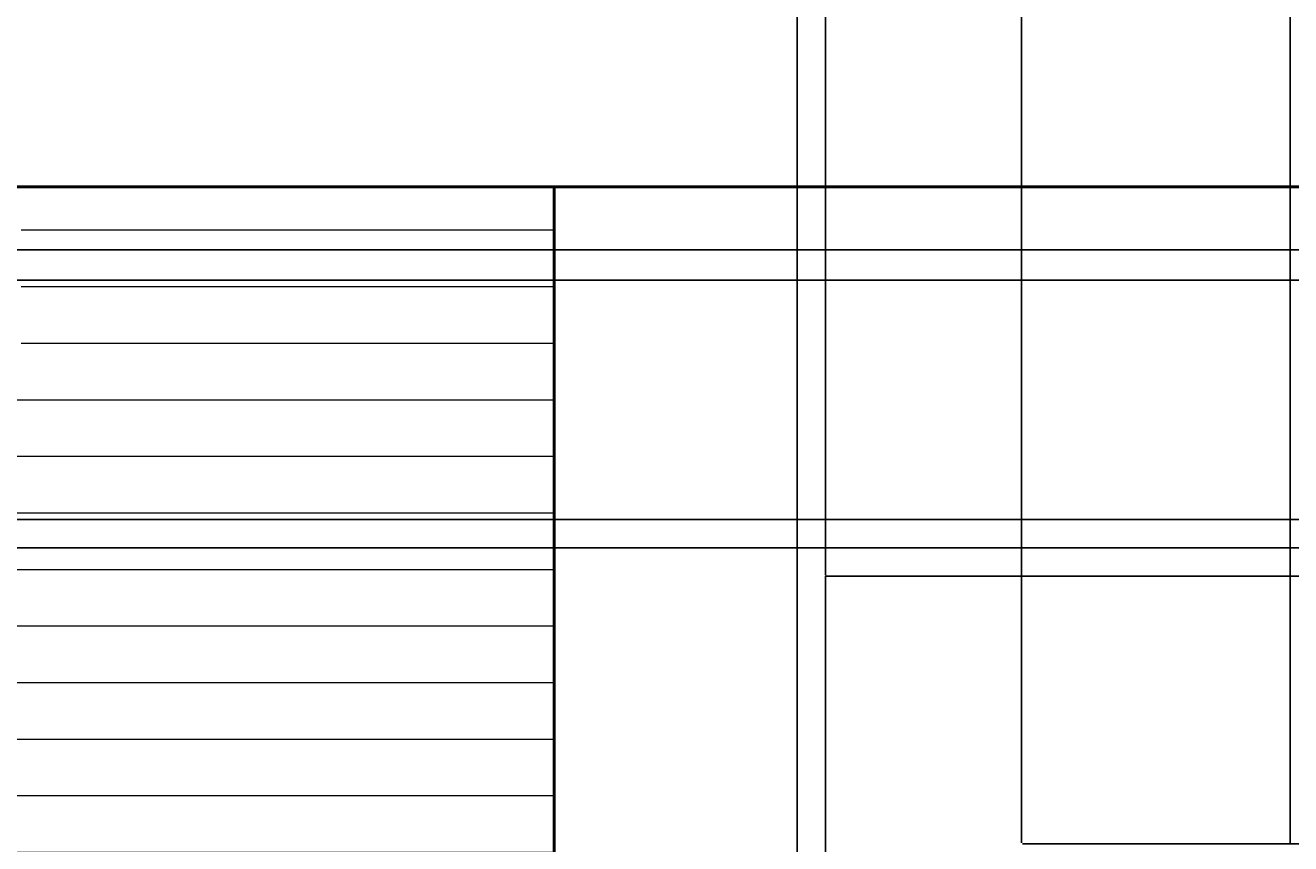
# Model space of a CAD drawing. Units: inches. Extents: x -139 to 346, y 72 to 413.
# Tile 12 of 18: x 175 to 265, y 185 to 242. Entities that reach past the tile are written whole.
import ezdxf

# ---------------------------------------------------------------- set-up
doc = ezdxf.new("R2010")
doc.units = ezdxf.units.IN
doc.header["$MEASUREMENT"] = 0
for name, color, linetype, lineweight in [('A-ANNO-DIMS', 2, 'Continuous', 18), ('A-DOOR', 3, 'Continuous', 25), ('A-WALL', 7, 'Continuous', 50), ('A-WALL-PATT', 8, 'Continuous', 13)]:
    doc.layers.add(name, color=color, linetype=linetype, lineweight=lineweight)
doc.styles.get("Standard").update_dxf_attribs({"font": 'arial.ttf'})
doc.dimstyles.get("Standard").update_dxf_attribs({"dimtxt": 0.6875, "dimasz": 0.18, "dimexe": 0.18, "dimexo": 0.0625, "dimgap": 0.09, "dimtad": 0, "dimtih": 1, "dimtoh": 1, "dimdec": 4, "dimzin": 0, "dimdsep": 46, "dimlunit": 4, "dimtxsty": 'Standard', "dimcen": 0.09, "dimadec": 0, "dimazin": 0, "dimtfac": 1, "dimtdec": 4, "dimtofl": 0, "dimtmove": 0, "dimatfit": 3, "dimfxl": 1, "dimtolj": 1, "dimtzin": 0, "dimarcsym": 0})

# ---------------------------------------------------------------- blocks, each defined once
blk = doc.blocks.new('*D54')
at = {"layer": 'A-ANNO-DIMS', "color": 0, "lineweight": -2, "transparency": 16777216}
for p, q in [((-47.211, 224.459), (344.386, 224.459)), ((344.206, 224.279), (344.206, 216.433)), ((344.206, 207.704), (344.206, 215.55)), ((-47.211, 207.524), (344.386, 207.524))]:
    blk.add_line(p, q, dxfattribs=at)
at = {"layer": 'A-ANNO-DIMS', "color": 0, "transparency": 16777216}
for points in [[(344.176, 224.279), (344.236, 224.279), (344.206, 224.459)], [(344.176, 207.704), (344.236, 207.704), (344.206, 207.524)]]:
    blk.add_solid(points, dxfattribs=at)
at = {"layer": 'Defpoints', "color": 0, "transparency": 16777216}
for p in [(-47.273, 224.459), (344.206, 224.459), (-47.273, 207.524)]:
    blk.add_point(p, dxfattribs=at)
at = {"layer": 'A-ANNO-DIMS', "color": 0, "transparency": 16777216, "insert": (344.206, 215.992), "char_height": 0.6875, "attachment_point": 5}
blk.add_mtext('\\A1;16.935', dxfattribs=at)
blk = doc.blocks.new('*D55')
at = {"layer": 'A-ANNO-DIMS', "color": 0, "lineweight": -2, "transparency": 16777216}
for p, q in [((-47.211, 226.606), (344.386, 226.606)), ((344.206, 226.426), (344.206, 225.968)), ((344.206, 224.639), (344.206, 225.097)), ((-47.211, 224.459), (344.386, 224.459))]:
    blk.add_line(p, q, dxfattribs=at)
at = {"layer": 'A-ANNO-DIMS', "color": 0, "transparency": 16777216}
for points in [[(344.176, 226.426), (344.236, 226.426), (344.206, 226.606)], [(344.176, 224.639), (344.236, 224.639), (344.206, 224.459)]]:
    blk.add_solid(points, dxfattribs=at)
at = {"layer": 'Defpoints', "color": 0, "transparency": 16777216}
for p in [(-47.273, 226.606), (344.206, 226.606), (-47.273, 224.459)]:
    blk.add_point(p, dxfattribs=at)
at = {"layer": 'A-ANNO-DIMS', "color": 0, "transparency": 16777216, "insert": (344.206, 225.533), "char_height": 0.6875, "attachment_point": 5}
blk.add_mtext('\\A1;2.147', dxfattribs=at)
blk = doc.blocks.new('*D65')
at = {"layer": 'A-ANNO-DIMS', "color": 0, "lineweight": -2, "transparency": 16777216}
for p, q in [((55.328, 205.524), (344.386, 205.524)), ((344.206, 205.344), (344.206, 178.581)), ((344.206, 150.938), (344.206, 177.701)), ((55.328, 150.758), (344.386, 150.758))]:
    blk.add_line(p, q, dxfattribs=at)
at = {"layer": 'A-ANNO-DIMS', "color": 0, "transparency": 16777216}
for points in [[(344.176, 205.344), (344.236, 205.344), (344.206, 205.524)], [(344.176, 150.938), (344.236, 150.938), (344.206, 150.758)]]:
    blk.add_solid(points, dxfattribs=at)
at = {"layer": 'Defpoints', "color": 0, "transparency": 16777216}
for p in [(55.265, 205.524), (344.206, 205.524), (55.265, 150.758)]:
    blk.add_point(p, dxfattribs=at)
at = {"layer": 'A-ANNO-DIMS', "color": 0, "transparency": 16777216, "insert": (344.206, 178.141), "char_height": 0.6875, "attachment_point": 5}
blk.add_mtext('\\A1;54.77', dxfattribs=at)
blk = doc.blocks.new('*D66')
at = {"layer": 'A-ANNO-DIMS', "color": 0, "lineweight": -2, "transparency": 16777216}
for p, q in [((57.328, 207.524), (344.386, 207.524)), ((344.206, 207.344), (344.206, 206.96)), ((344.206, 205.704), (344.206, 206.089)), ((55.328, 205.524), (344.386, 205.524))]:
    blk.add_line(p, q, dxfattribs=at)
at = {"layer": 'A-ANNO-DIMS', "color": 0, "transparency": 16777216}
for points in [[(344.176, 207.344), (344.236, 207.344), (344.206, 207.524)], [(344.176, 205.704), (344.236, 205.704), (344.206, 205.524)]]:
    blk.add_solid(points, dxfattribs=at)
at = {"layer": 'Defpoints', "color": 0, "transparency": 16777216}
for p in [(57.265, 207.524), (344.206, 207.524), (55.265, 205.524)]:
    blk.add_point(p, dxfattribs=at)
at = {"layer": 'A-ANNO-DIMS', "color": 0, "transparency": 16777216, "insert": (344.206, 206.524), "char_height": 0.6875, "attachment_point": 5}
blk.add_mtext('\\A1;2', dxfattribs=at)
blk = doc.blocks.new('*D67')
at = {"layer": 'A-ANNO-DIMS', "color": 0, "lineweight": -2, "transparency": 16777216}
for p, q in [((57.328, 207.524), (344.386, 207.524)), ((344.206, 207.344), (344.206, 165.091)), ((344.206, 121.955), (344.206, 164.209)), ((57.328, 121.775), (344.386, 121.775))]:
    blk.add_line(p, q, dxfattribs=at)
at = {"layer": 'A-ANNO-DIMS', "color": 0, "transparency": 16777216}
for points in [[(344.176, 207.344), (344.236, 207.344), (344.206, 207.524)], [(344.176, 121.955), (344.236, 121.955), (344.206, 121.775)]]:
    blk.add_solid(points, dxfattribs=at)
at = {"layer": 'Defpoints', "color": 0, "transparency": 16777216}
for p in [(57.265, 207.524), (344.206, 207.524), (57.265, 121.775)]:
    blk.add_point(p, dxfattribs=at)
at = {"layer": 'A-ANNO-DIMS', "color": 0, "transparency": 16777216, "insert": (344.206, 164.65), "char_height": 0.6875, "attachment_point": 5}
blk.add_mtext('\\A1;85.75', dxfattribs=at)
blk = doc.blocks.new('*D80')
at = {"layer": 'A-ANNO-DIMS', "color": 0, "lineweight": -2, "transparency": 16777216}
for p, q in [((229.972, 205.587), (229.972, 412.455)), ((230.152, 412.275), (230.654, 412.275)), ((231.792, 412.275), (231.29, 412.275)), ((231.972, 203.587), (231.972, 412.455))]:
    blk.add_line(p, q, dxfattribs=at)
at = {"layer": 'A-ANNO-DIMS', "color": 0, "transparency": 16777216}
for points in [[(230.152, 412.305), (230.152, 412.245), (229.972, 412.275)], [(231.792, 412.305), (231.792, 412.245), (231.972, 412.275)]]:
    blk.add_solid(points, dxfattribs=at)
at = {"layer": 'Defpoints', "color": 0, "transparency": 16777216}
for p in [(231.972, 412.275), (229.972, 205.524), (231.972, 203.524)]:
    blk.add_point(p, dxfattribs=at)
at = {"layer": 'A-ANNO-DIMS', "color": 0, "transparency": 16777216, "insert": (230.972, 412.275), "char_height": 0.6875, "attachment_point": 5}
blk.add_mtext('\\A1;2', dxfattribs=at)
blk = doc.blocks.new('*D81')
at = {"layer": 'A-ANNO-DIMS', "color": 0, "lineweight": -2, "transparency": 16777216}
for p, q in [((231.972, 203.587), (231.972, 412.455)), ((232.152, 412.275), (237.421, 412.275)), ((245.66, 412.275), (240.391, 412.275)), ((245.84, 184.668), (245.84, 412.455))]:
    blk.add_line(p, q, dxfattribs=at)
at = {"layer": 'A-ANNO-DIMS', "color": 0, "transparency": 16777216}
for points in [[(232.152, 412.305), (232.152, 412.245), (231.972, 412.275)], [(245.66, 412.305), (245.66, 412.245), (245.84, 412.275)]]:
    blk.add_solid(points, dxfattribs=at)
at = {"layer": 'Defpoints', "color": 0, "transparency": 16777216}
for p in [(245.84, 412.275), (231.972, 203.524), (245.84, 184.606)]:
    blk.add_point(p, dxfattribs=at)
at = {"layer": 'A-ANNO-DIMS', "color": 0, "transparency": 16777216, "insert": (238.906, 412.275), "char_height": 0.6875, "attachment_point": 5}
blk.add_mtext('\\A1;13.868', dxfattribs=at)
blk = doc.blocks.new('*D82')
at = {"layer": 'A-ANNO-DIMS', "color": 0, "lineweight": -2, "transparency": 16777216}
for p, q in [((245.84, 184.668), (245.84, 412.455)), ((246.02, 412.275), (253.85, 412.275)), ((264.642, 412.275), (256.812, 412.275)), ((264.822, 184.668), (264.822, 412.455))]:
    blk.add_line(p, q, dxfattribs=at)
at = {"layer": 'A-ANNO-DIMS', "color": 0, "transparency": 16777216}
for points in [[(246.02, 412.305), (246.02, 412.245), (245.84, 412.275)], [(264.642, 412.305), (264.642, 412.245), (264.822, 412.275)]]:
    blk.add_solid(points, dxfattribs=at)
at = {"layer": 'Defpoints', "color": 0, "transparency": 16777216}
for p in [(264.822, 412.275), (245.84, 184.606), (264.822, 184.606)]:
    blk.add_point(p, dxfattribs=at)
at = {"layer": 'A-ANNO-DIMS', "color": 0, "transparency": 16777216, "insert": (255.331, 412.275), "char_height": 0.6875, "attachment_point": 5}
blk.add_mtext('\\A1;18.982', dxfattribs=at)
blk = doc.blocks.new('*D84')
at = {"layer": 'A-ANNO-DIMS', "color": 0, "lineweight": -2, "transparency": 16777216}
for p, q in [((245.902, 184.606), (344.386, 184.606)), ((344.206, 184.426), (344.206, 153.665)), ((344.206, 122.023), (344.206, 152.783)), ((245.902, 121.843), (344.386, 121.843))]:
    blk.add_line(p, q, dxfattribs=at)
at = {"layer": 'A-ANNO-DIMS', "color": 0, "transparency": 16777216}
for points in [[(344.176, 184.426), (344.236, 184.426), (344.206, 184.606)], [(344.176, 122.023), (344.236, 122.023), (344.206, 121.843)]]:
    blk.add_solid(points, dxfattribs=at)
at = {"layer": 'Defpoints', "color": 0, "transparency": 16777216}
for p in [(245.84, 184.606), (344.206, 184.606), (245.84, 121.843)]:
    blk.add_point(p, dxfattribs=at)
at = {"layer": 'A-ANNO-DIMS', "color": 0, "transparency": 16777216, "insert": (344.206, 153.224), "char_height": 0.6875, "attachment_point": 5}
blk.add_mtext('\\A1;62.76', dxfattribs=at)

msp = doc.modelspace()

# ---------------------------------------------------------------- hatches: boundary and pattern name
at = {"layer": 'A-WALL-PATT'}
h = msp.add_hatch(dxfattribs=at)
h.set_pattern_fill('ANSI31', color=256, scale=32, angle=135)
h.paths.add_polyline_path([(98.6724, 360.5443), (-34.7346, 360.5443), (-34.7346, 353.0644), (-34.7346, 305.9205), (5.6729, 305.9205), (5.6729, 338.3217), (62.4258, 338.3217), (62.4258, 305.9205), (98.6724, 305.9205)])
h.paths.add_polyline_path([(212.769, 231.0607), (175.072, 231.0607), (175.072, 218.0635), (171.0337, 218.0635), (171.0337, 115.6761), (125.2464, 115.6761), (125.2464, 218.0635), (123.4318, 218.0635), (120.5054, 218.0635), (120.5054, 231.0607), (112.6506, 231.0607), (112.6506, 112.6042), (212.769, 112.6042)])

# ---------------------------------------------------------------- linework, layer by layer
at = {"layer": 'A-DOOR'}
for points in [[(229.972, 205.5243), (283.8497, 205.5243), (283.8497, 104.5429), (229.972, 104.5429)], [(231.972, 203.5243), (281.8497, 203.5243), (281.8497, 106.5429), (231.972, 106.5429)]]:
    msp.add_lwpolyline(points, close=True, dxfattribs=at)
at = {"layer": 'A-WALL'}
for p, q in [((297.5013, 231.0607), (112.6506, 231.0607)), ((212.769, 231.0607), (212.769, 94.9748))]:
    msp.add_line(p, q, dxfattribs=at)

# ---------------------------------------------------------------- dimensions: what is measured, and where the dimension line sits
at = {"layer": 'A-ANNO-DIMS'}
for base, p1, p2, override, picture, middle in [((231.972, 412.2748), (229.972, 205.5243), (231.972, 203.5243), {"dimdec": 0, "dimlfac": 1, "dimrnd": 0, "dimzin": 0, "dimdsep": 46, "dimlunit": 2}, '*D80', (230.972, 412.2748)), ((245.8399, 412.2748), (231.972, 203.5243), (245.8399, 184.6055), {"dimdec": 3, "dimlfac": 1, "dimrnd": 0, "dimzin": 0, "dimdsep": 46, "dimlunit": 2}, '*D81', (238.906, 412.2748)), ((264.8219, 412.2748), (245.8399, 184.6055), (264.8219, 184.6055), {"dimdec": 3, "dimlfac": 1, "dimrnd": 0, "dimzin": 0, "dimdsep": 46, "dimlunit": 2}, '*D82', (255.3309, 412.2748))]:
    dim = msp.add_linear_dim(base=base, p1=p1, p2=p2, dimstyle='Standard', override=override, dxfattribs=at)
    dim.commit()
    dim.dimension.update_dxf_attribs({"geometry": picture, "text_midpoint": middle})
for base, p1, p2, override, picture, middle in [((344.2055, 226.6062), (-47.2734, 224.4591), (-47.2734, 226.6062), {"dimdec": 3, "dimlfac": 1, "dimrnd": 0, "dimzin": 0, "dimdsep": 46, "dimlunit": 2}, '*D55', (344.2055, 225.5327)), ((344.2055, 224.4591), (-47.2734, 207.5243), (-47.2734, 224.4591), {"dimdec": 3, "dimlfac": 1, "dimrnd": 0, "dimzin": 0, "dimdsep": 46, "dimlunit": 2}, '*D54', (344.2055, 215.9917)), ((344.2055, 207.5243), (55.2654, 205.5243), (57.2654, 207.5243), {"dimdec": 0, "dimlfac": 1, "dimrnd": 0, "dimzin": 0, "dimdsep": 46, "dimlunit": 2}, '*D66', (344.2055, 206.5243)), ((344.2055, 207.5243), (57.2654, 121.7753), (57.2654, 207.5243), {"dimdec": 2, "dimlfac": 1, "dimrnd": 0, "dimzin": 0, "dimdsep": 46, "dimlunit": 2}, '*D67', (344.2055, 164.6498)), ((344.2055, 205.5243), (55.2654, 150.7576), (55.2654, 205.5243), {"dimdec": 2, "dimlfac": 1, "dimrnd": 0, "dimzin": 0, "dimdsep": 46, "dimlunit": 2}, '*D65', (344.2055, 178.141)), ((344.2055, 184.6055), (245.8399, 121.8428), (245.8399, 184.6055), {"dimdec": 2, "dimlfac": 1, "dimrnd": 0, "dimzin": 0, "dimdsep": 46, "dimlunit": 2}, '*D84', (344.2055, 153.2242))]:
    dim = msp.add_linear_dim(base=base, p1=p1, p2=p2, angle=90, dimstyle='Standard', override=override, dxfattribs=at)
    dim.commit()
    dim.dimension.update_dxf_attribs({"geometry": picture, "text_midpoint": middle})

doc.saveas('drawing.dxf')
